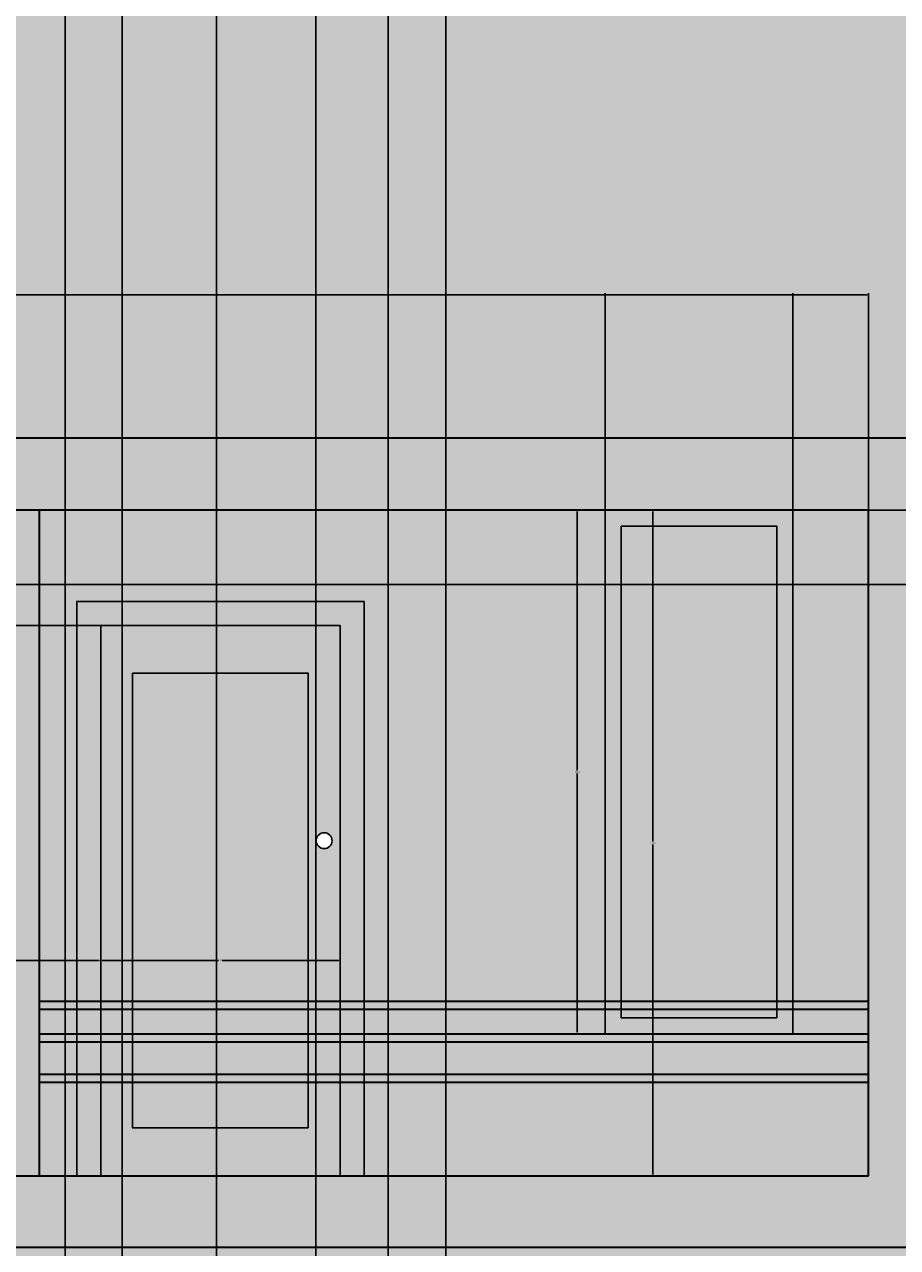
# Model space of a CAD drawing. Units: inches. Extents: x 73 to 607, y 92 to 651.
# Tile 15 of 18: x 337 to 446, y 311 to 465. Entities that reach past the tile are written whole.
import ezdxf

# ---------------------------------------------------------------- set-up
doc = ezdxf.new("R2010")
doc.units = ezdxf.units.IN
doc.header["$MEASUREMENT"] = 0
for name, color, linetype, lineweight in [('A-ANNO-DIMS', 2, 'Continuous', 18), ('A-DOOR', 3, 'Continuous', 25), ('A-ELEV', 7, 'Continuous', 35), ('A-ELEV-PATT-BKGD', 252, 'Continuous', 13), ('A-ELEV-PATT-FRAM', 38, 'Continuous', 13), ('A-ELEV-PATT-SHAD', 8, 'Continuous', 13), ('A-ELEV-PATT-WALL', 254, 'Continuous', 13), ('A-GLAZ', 4, 'Continuous', 25), ('A-GLAZ-PATT', 7, 'Continuous', 13)]:
    doc.layers.add(name, color=color, linetype=linetype, lineweight=lineweight)
doc.styles.get("Standard").update_dxf_attribs({"font": 'arial.ttf'})
doc.dimstyles.get("Standard").update_dxf_attribs({"dimtxt": 0.18, "dimasz": 0.18, "dimexe": 0.18, "dimexo": 0.0625, "dimgap": 0.09, "dimtad": 0, "dimtih": 1, "dimtoh": 1, "dimdec": 4, "dimzin": 0, "dimdsep": 46, "dimtxsty": 'Standard', "dimcen": 0.09, "dimadec": 0, "dimazin": 0, "dimtfac": 1, "dimtdec": 4, "dimtofl": 0, "dimtmove": 0, "dimatfit": 3, "dimfxl": 1, "dimtolj": 1, "dimtzin": 0, "dimarcsym": 0})

# ---------------------------------------------------------------- blocks, each defined once
blk = doc.blocks.new('*U3')
blk.add_lwpolyline([(3.12, 0.01), (0.12, 0.01), (0.12, 72.01), (36.12, 72.01), (36.12, 0.01), (33.12, 0.01)])
for points in [[(33.12, 68.99), (33.12, 0.01), (3.12, 0.01), (3.12, 68.99)], [(29.12, 6.01), (29.12, 62.99), (7.12, 62.99), (7.12, 6.01)]]:
    blk.add_lwpolyline(points, close=True)
blk.add_circle((31.12, 42.01), 1)
blk = doc.blocks.new('*D52')
at = {"layer": 'A-ANNO-DIMS', "color": 0, "lineweight": -2, "transparency": 16777216}
for p, q in [((206.13, 403.7), (206.13, 430.82)), ((442.52, 403.7), (442.52, 430.82)), ((206.31, 430.64), (323.93, 430.64)), ((442.34, 430.64), (324.72, 430.64))]:
    blk.add_line(p, q, dxfattribs=at)
at = {"layer": 'A-ANNO-DIMS', "color": 0, "transparency": 16777216}
for points in [[(206.31, 430.67), (206.31, 430.61), (206.13, 430.64)], [(442.34, 430.67), (442.34, 430.61), (442.52, 430.64)]]:
    blk.add_solid(points, dxfattribs=at)
at = {"layer": 'Defpoints', "color": 0, "transparency": 16777216}
for p in [(442.52, 430.64), (206.13, 403.64), (442.52, 403.64)]:
    blk.add_point(p, dxfattribs=at)
at = {"layer": 'A-ANNO-DIMS', "color": 0, "transparency": 16777216, "insert": (324.33, 430.64), "char_height": 0.18, "attachment_point": 5}
blk.add_mtext('\\A1;236.4', dxfattribs=at)
blk = doc.blocks.new('*D53')
at = {"layer": 'A-ANNO-DIMS', "color": 0, "lineweight": -2, "transparency": 16777216}
for p, q in [((442.46, 403.64), (415.34, 403.64)), ((415.52, 403.46), (415.52, 362.1)), ((415.52, 320.38), (415.52, 361.74)), ((442.46, 320.2), (415.34, 320.2))]:
    blk.add_line(p, q, dxfattribs=at)
at = {"layer": 'A-ANNO-DIMS', "color": 0, "transparency": 16777216}
for points in [[(415.49, 403.46), (415.55, 403.46), (415.52, 403.64)], [(415.49, 320.38), (415.55, 320.38), (415.52, 320.2)]]:
    blk.add_solid(points, dxfattribs=at)
at = {"layer": 'Defpoints', "color": 0, "transparency": 16777216}
for p in [(415.52, 403.64), (442.52, 403.64), (442.52, 320.2)]:
    blk.add_point(p, dxfattribs=at)
at = {"layer": 'A-ANNO-DIMS', "color": 0, "transparency": 16777216, "insert": (415.52, 361.92), "char_height": 0.18, "attachment_point": 5}
blk.add_mtext('\\A1;83.43', dxfattribs=at)
blk = doc.blocks.new('*D54')
at = {"layer": 'A-ANNO-DIMS', "color": 0, "lineweight": -2, "transparency": 16777216}
for p, q in [((206.13, 320.27), (206.13, 347.38)), ((206.31, 347.2), (275.84, 347.2)), ((346.14, 347.2), (276.61, 347.2)), ((346.32, 320.27), (346.32, 347.38))]:
    blk.add_line(p, q, dxfattribs=at)
at = {"layer": 'A-ANNO-DIMS', "color": 0, "transparency": 16777216}
for points in [[(206.31, 347.23), (206.31, 347.17), (206.13, 347.2)], [(346.14, 347.23), (346.14, 347.17), (346.32, 347.2)]]:
    blk.add_solid(points, dxfattribs=at)
at = {"layer": 'Defpoints', "color": 0, "transparency": 16777216}
for p in [(346.32, 347.2), (206.13, 320.2), (346.32, 320.2)]:
    blk.add_point(p, dxfattribs=at)
at = {"layer": 'A-ANNO-DIMS', "color": 0, "transparency": 16777216, "insert": (276.23, 347.2), "char_height": 0.18, "attachment_point": 5}
blk.add_mtext('\\A1;140.2', dxfattribs=at)
blk = doc.blocks.new('*D55')
at = {"layer": 'A-ANNO-DIMS', "color": 0, "lineweight": -2, "transparency": 16777216}
for p, q in [((346.32, 320.27), (346.32, 347.38)), ((346.5, 347.2), (361.1, 347.2)), ((376.14, 347.2), (361.54, 347.2)), ((376.32, 320.27), (376.32, 347.38))]:
    blk.add_line(p, q, dxfattribs=at)
at = {"layer": 'A-ANNO-DIMS', "color": 0, "transparency": 16777216}
for points in [[(346.5, 347.23), (346.5, 347.17), (346.32, 347.2)], [(376.14, 347.23), (376.14, 347.17), (376.32, 347.2)]]:
    blk.add_solid(points, dxfattribs=at)
at = {"layer": 'Defpoints', "color": 0, "transparency": 16777216}
for p in [(376.32, 347.2), (346.32, 320.2), (376.32, 320.2)]:
    blk.add_point(p, dxfattribs=at)
at = {"layer": 'A-ANNO-DIMS', "color": 0, "transparency": 16777216, "insert": (361.32, 347.2), "char_height": 0.18, "attachment_point": 5}
blk.add_mtext('\\A1;30', dxfattribs=at)
blk = doc.blocks.new('*D56')
at = {"layer": 'A-ANNO-DIMS', "color": 0, "lineweight": -2, "transparency": 16777216}
for p, q in [((346.26, 389.18), (319.14, 389.18)), ((319.32, 389), (319.32, 354.87)), ((319.32, 320.38), (319.32, 354.51)), ((346.26, 320.2), (319.14, 320.2))]:
    blk.add_line(p, q, dxfattribs=at)
at = {"layer": 'A-ANNO-DIMS', "color": 0, "transparency": 16777216}
for points in [[(319.29, 389), (319.35, 389), (319.32, 389.18)], [(319.29, 320.38), (319.35, 320.38), (319.32, 320.2)]]:
    blk.add_solid(points, dxfattribs=at)
at = {"layer": 'Defpoints', "color": 0, "transparency": 16777216}
for p in [(319.32, 389.18), (346.32, 389.18), (346.32, 320.2)]:
    blk.add_point(p, dxfattribs=at)
at = {"layer": 'A-ANNO-DIMS', "color": 0, "transparency": 16777216, "insert": (319.32, 354.69), "char_height": 0.18, "attachment_point": 5}
blk.add_mtext('\\A1;68.98', dxfattribs=at)
blk = doc.blocks.new('*D57')
at = {"layer": 'A-ANNO-DIMS', "color": 0, "lineweight": -2, "transparency": 16777216}
for p, q in [((409.52, 403.7), (409.52, 430.82)), ((433.03, 403.7), (433.03, 430.82)), ((409.7, 430.64), (420.89, 430.64)), ((432.85, 430.64), (421.65, 430.64))]:
    blk.add_line(p, q, dxfattribs=at)
at = {"layer": 'A-ANNO-DIMS', "color": 0, "transparency": 16777216}
for points in [[(409.7, 430.67), (409.7, 430.61), (409.52, 430.64)], [(432.85, 430.67), (432.85, 430.61), (433.03, 430.64)]]:
    blk.add_solid(points, dxfattribs=at)
at = {"layer": 'Defpoints', "color": 0, "transparency": 16777216}
for p in [(433.03, 430.64), (409.52, 403.64), (433.03, 403.64)]:
    blk.add_point(p, dxfattribs=at)
at = {"layer": 'A-ANNO-DIMS', "color": 0, "transparency": 16777216, "insert": (421.27, 430.64), "char_height": 0.18, "attachment_point": 5}
blk.add_mtext('\\A1;23.51', dxfattribs=at)
blk = doc.blocks.new('*D58')
at = {"layer": 'A-ANNO-DIMS', "color": 0, "lineweight": -2, "transparency": 16777216}
for p, q in [((432.96, 403.64), (405.85, 403.64)), ((406.03, 403.46), (406.03, 371)), ((406.03, 338.18), (406.03, 370.64)), ((432.96, 338), (405.85, 338))]:
    blk.add_line(p, q, dxfattribs=at)
at = {"layer": 'A-ANNO-DIMS', "color": 0, "transparency": 16777216}
for points in [[(406, 403.46), (406.06, 403.46), (406.03, 403.64)], [(406, 338.18), (406.06, 338.18), (406.03, 338)]]:
    blk.add_solid(points, dxfattribs=at)
at = {"layer": 'Defpoints', "color": 0, "transparency": 16777216}
for p in [(406.03, 403.64), (433.03, 403.64), (433.03, 338)]:
    blk.add_point(p, dxfattribs=at)
at = {"layer": 'A-ANNO-DIMS', "color": 0, "transparency": 16777216, "insert": (406.03, 370.82), "char_height": 0.18, "attachment_point": 5}
blk.add_mtext('\\A1;65.63', dxfattribs=at)
blk = doc.blocks.new('*D79')
at = {"layer": 'A-ANNO-DIMS', "color": 0, "lineweight": -2, "transparency": 16777216}
for p, q in [((334.73, 403.64), (607.28, 403.64)), ((607.1, 403.46), (607.1, 399.16)), ((607.1, 394.49), (607.1, 398.79)), ((316.35, 394.31), (607.28, 394.31))]:
    blk.add_line(p, q, dxfattribs=at)
at = {"layer": 'A-ANNO-DIMS', "color": 0, "transparency": 16777216}
for points in [[(607.07, 403.46), (607.13, 403.46), (607.1, 403.64)], [(607.07, 394.49), (607.13, 394.49), (607.1, 394.31)]]:
    blk.add_solid(points, dxfattribs=at)
at = {"layer": 'Defpoints', "color": 0, "transparency": 16777216}
for p in [(334.67, 403.64), (316.28, 394.31), (607.1, 394.31)]:
    blk.add_point(p, dxfattribs=at)
at = {"layer": 'A-ANNO-DIMS', "color": 0, "transparency": 16777216, "insert": (607.1, 398.98), "char_height": 0.18, "attachment_point": 5}
blk.add_mtext('\\A1;9.322', dxfattribs=at)
blk = doc.blocks.new('*D81')
at = {"layer": 'A-ANNO-DIMS', "color": 0, "lineweight": -2, "transparency": 16777216}
for p, q in [((341.87, 247.47), (341.87, 650.98)), ((342.05, 650.8), (345.04, 650.8)), ((348.82, 650.8), (345.83, 650.8)), ((349, 237.52), (349, 650.98))]:
    blk.add_line(p, q, dxfattribs=at)
at = {"layer": 'A-ANNO-DIMS', "color": 0, "transparency": 16777216}
for points in [[(342.05, 650.83), (342.05, 650.77), (341.87, 650.8)], [(348.82, 650.83), (348.82, 650.77), (349, 650.8)]]:
    blk.add_solid(points, dxfattribs=at)
at = {"layer": 'Defpoints', "color": 0, "transparency": 16777216}
for p in [(349, 650.8), (341.87, 247.41), (349, 237.45)]:
    blk.add_point(p, dxfattribs=at)
at = {"layer": 'A-ANNO-DIMS', "color": 0, "transparency": 16777216, "insert": (345.43, 650.8), "char_height": 0.18, "attachment_point": 5}
blk.add_mtext('\\A1;7.128', dxfattribs=at)
blk = doc.blocks.new('*D82')
at = {"layer": 'A-ANNO-DIMS', "color": 0, "lineweight": -2, "transparency": 16777216}
for p, q in [((349, 237.52), (349, 650.98)), ((349.18, 650.8), (354.47, 650.8)), ((360.67, 650.8), (355.38, 650.8)), ((360.85, 239), (360.85, 650.98))]:
    blk.add_line(p, q, dxfattribs=at)
at = {"layer": 'A-ANNO-DIMS', "color": 0, "transparency": 16777216}
for points in [[(349.18, 650.83), (349.18, 650.77), (349, 650.8)], [(360.67, 650.83), (360.67, 650.77), (360.85, 650.8)]]:
    blk.add_solid(points, dxfattribs=at)
at = {"layer": 'Defpoints', "color": 0, "transparency": 16777216}
for p in [(360.85, 650.8), (360.85, 238.93), (349, 237.45)]:
    blk.add_point(p, dxfattribs=at)
at = {"layer": 'A-ANNO-DIMS', "color": 0, "transparency": 16777216, "insert": (354.92, 650.8), "char_height": 0.18, "attachment_point": 5}
blk.add_mtext('\\A1;11.852', dxfattribs=at)
blk = doc.blocks.new('*D83')
at = {"layer": 'A-ANNO-DIMS', "color": 0, "lineweight": -2, "transparency": 16777216}
for p, q in [((360.85, 239), (360.85, 650.98)), ((361.03, 650.8), (366.6, 650.8)), ((373.08, 650.8), (367.51, 650.8)), ((373.26, 231.41), (373.26, 650.98))]:
    blk.add_line(p, q, dxfattribs=at)
at = {"layer": 'A-ANNO-DIMS', "color": 0, "transparency": 16777216}
for points in [[(361.03, 650.83), (361.03, 650.77), (360.85, 650.8)], [(373.08, 650.83), (373.08, 650.77), (373.26, 650.8)]]:
    blk.add_solid(points, dxfattribs=at)
at = {"layer": 'Defpoints', "color": 0, "transparency": 16777216}
for p in [(373.26, 650.8), (360.85, 238.93), (373.26, 231.35)]:
    blk.add_point(p, dxfattribs=at)
at = {"layer": 'A-ANNO-DIMS', "color": 0, "transparency": 16777216, "insert": (367.05, 650.8), "char_height": 0.18, "attachment_point": 5}
blk.add_mtext('\\A1;12.408', dxfattribs=at)
blk = doc.blocks.new('*D84')
at = {"layer": 'A-ANNO-DIMS', "color": 0, "lineweight": -2, "transparency": 16777216}
for p, q in [((373.26, 231.41), (373.26, 650.98)), ((373.44, 650.8), (377.4, 650.8)), ((382.15, 650.8), (378.19, 650.8)), ((382.33, 241.03), (382.33, 650.98))]:
    blk.add_line(p, q, dxfattribs=at)
at = {"layer": 'A-ANNO-DIMS', "color": 0, "transparency": 16777216}
for points in [[(373.44, 650.83), (373.44, 650.77), (373.26, 650.8)], [(382.15, 650.83), (382.15, 650.77), (382.33, 650.8)]]:
    blk.add_solid(points, dxfattribs=at)
at = {"layer": 'Defpoints', "color": 0, "transparency": 16777216}
for p in [(382.33, 650.8), (382.33, 240.97), (373.26, 231.35)]:
    blk.add_point(p, dxfattribs=at)
at = {"layer": 'A-ANNO-DIMS', "color": 0, "transparency": 16777216, "insert": (377.79, 650.8), "char_height": 0.18, "attachment_point": 5}
blk.add_mtext('\\A1;9.074', dxfattribs=at)
blk = doc.blocks.new('*D85')
at = {"layer": 'A-ANNO-DIMS', "color": 0, "lineweight": -2, "transparency": 16777216}
for p, q in [((382.33, 241.03), (382.33, 650.98)), ((382.51, 650.8), (385.55, 650.8)), ((389.37, 650.8), (386.33, 650.8)), ((389.55, 232.52), (389.55, 650.98))]:
    blk.add_line(p, q, dxfattribs=at)
at = {"layer": 'A-ANNO-DIMS', "color": 0, "transparency": 16777216}
for points in [[(382.51, 650.83), (382.51, 650.77), (382.33, 650.8)], [(389.37, 650.83), (389.37, 650.77), (389.55, 650.8)]]:
    blk.add_solid(points, dxfattribs=at)
at = {"layer": 'Defpoints', "color": 0, "transparency": 16777216}
for p in [(389.55, 650.8), (382.33, 240.97), (389.55, 232.46)]:
    blk.add_point(p, dxfattribs=at)
at = {"layer": 'A-ANNO-DIMS', "color": 0, "transparency": 16777216, "insert": (385.94, 650.8), "char_height": 0.18, "attachment_point": 5}
blk.add_mtext('\\A1;7.222', dxfattribs=at)

msp = doc.modelspace()

# ---------------------------------------------------------------- hatches: boundary and pattern name
at = {"layer": 'A-ELEV-PATT-BKGD'}
h = msp.add_hatch(color=256, dxfattribs=at)
h.dxf.hatch_style = 1
h.paths.add_polyline_path([(321.3008, 479.2042), (312.3008, 479.2042), (312.3008, 478.7576), (312.3008, 412.636), (321.3008, 412.636)])
h.paths.add_polyline_path([(312.3008, 504.7576), (256.4726, 504.7576), (256.4726, 503.4576), (312.3008, 503.4576)], flags=17)
h.paths.add_polyline_path([(321.3008, 543.1576), (321.3008, 552.1576), (320.3257, 552.1576), (312.3008, 552.1576), (256.4726, 552.1576), (256.4726, 543.1576), (312.3008, 543.1576), (312.3008, 479.2042), (321.3008, 479.2042)])
h.paths.add_polyline_path([(451.5214, 412.636), (256.4726, 412.636), (256.4726, 403.636), (442.5214, 403.636), (442.5214, 320.2042), (206.1343, 320.2042), (206.1343, 320.9135), (206.1343, 403.636), (256.4726, 403.636), (256.4726, 412.636), (201.6343, 412.636), (201.6343, 320.9135), (201.6343, 320.2042), (201.6343, 311.2042), (256.4726, 311.2042), (451.5214, 311.2042)])
h.paths.add_polyline_path([(431.07, 258.6914), (369.5339, 258.6914), (369.5339, 247.4054), (396.692, 247.4054), (425.07, 247.4054), (425.07, 194.7312), (396.692, 194.6197), (396.692, 194.5366), (369.5339, 194.5366), (369.5339, 185.6619), (431.07, 185.6619)])
h.paths.add_polyline_path([(580.0983, 262.3024), (451.5214, 262.3024), (451.5214, 143.2042), (580.0983, 143.2042)])
h.paths.add_polyline_path([(454.7049, 174.802), (454.7049, 256.6321), (577.9249, 256.6321), (577.9249, 174.802)], flags=16)
h.paths.add_polyline_path([(465.9716, 191.1416, -1), (473.7874, 191.1416, -1)], flags=0)
h.paths.add_polyline_path([(490.5373, 181.6586, -1), (494.9999, 181.6586, -1)], flags=0)
h.paths.add_polyline_path([(476.2996, 209.8287, -1), (500.5844, 209.8287, -1)], flags=0)
h.paths.add_polyline_path([(505.3326, 194.7675, -1), (512.5843, 194.7675, -1)], flags=0)
h.paths.add_polyline_path([(520.9613, 186.679, -1), (526.544, 186.679, -1)], flags=0)
h.paths.add_polyline_path([(466.8103, 225.7267, -1), (470.1573, 225.7267, -1)], flags=0)
h.paths.add_polyline_path([(527.1059, 203.6926, -1), (536.0311, 203.6926, -1)], flags=0)
h.paths.add_polyline_path([(504.775, 232.6995, -1), (513.7002, 232.6995, -1)], flags=0)
h.paths.add_polyline_path([(546.9241, 183.611, -1), (554.7336, 183.611, -1)], flags=0)
h.paths.add_polyline_path([(459.5544, 243.856, -1), (466.8061, 243.856, -1)], flags=0)
h.paths.add_polyline_path([(476.3045, 246.924, -1), (488.5767, 246.924, -1)], flags=0)
h.paths.add_polyline_path([(529.9044, 226.8424, -1), (556.68, 226.8424, -1)], flags=0)
h.paths.add_polyline_path([(554.1814, 203.9716, -1), (561.4331, 203.9716, -1)], flags=0)
h.paths.add_polyline_path([(567.8561, 193.3729, -1), (570.6475, 193.3729, -1)], flags=0)
h.paths.add_polyline_path([(522.3584, 250.271, -1), (525.7053, 250.271, -1)], flags=0)
h.paths.add_polyline_path([(561.9965, 245.2506, -1), (567.5748, 245.2506, -1)], flags=0)
h.paths.add_polyline_path([(347.8686, 194.5366), (341.8686, 194.5366), (341.8686, 194.5452), (314.0144, 194.5452), (314.0144, 188.5452), (347.8686, 188.5452)])
h.paths.add_polyline_path([(347.8686, 253.4054), (314.0144, 253.4054), (314.0144, 247.4054), (341.8686, 247.4054), (347.8686, 247.4054)])
h.paths.add_polyline_path([(304.3559, 253.4054), (298.3559, 253.4054), (298.3559, 188.5452), (304.3559, 188.5452)])
h.paths.add_polyline_path([(450.6603, 552.1576), (369.9727, 552.1576), (369.9727, 479.2042), (374.4727, 479.2042), (374.4727, 547.6576), (446.1603, 547.6576), (446.1603, 479.2042), (450.6603, 479.2042)])
h.paths.add_polyline_path([(374.4727, 479.2042), (369.9727, 479.2042), (369.9727, 465.0632), (374.4727, 465.0632)])
h.paths.add_polyline_path([(450.6603, 479.2042), (446.1603, 479.2042), (446.1603, 465.0632), (450.6603, 465.0632)])
h.paths.add_polyline_path([(256.4726, 281.6039), (109.0983, 281.6039), (100.0983, 281.6039), (100.0983, 167.2042), (100.0983, 143.2042), (109.0983, 143.2042), (109.0983, 167.2042), (109.0983, 272.6039), (256.4726, 272.6039)])
at = {"layer": 'A-ELEV-PATT-FRAM'}
h = msp.add_hatch(color=256, dxfattribs=at)
h.dxf.hatch_style = 1
h.paths.add_polyline_path([(433.025, 403.636), (409.515, 403.636), (409.515, 342.1009), (411.515, 342.1009), (411.515, 401.636), (431.025, 401.636), (431.025, 342.1009), (433.025, 342.1009)])
h.paths.add_polyline_path([(433.025, 341.1009), (431.025, 341.1009), (431.025, 340.0025), (411.515, 340.0025), (411.515, 341.1009), (409.515, 341.1009), (409.515, 338.0025), (433.025, 338.0025)])
h.paths.add_polyline_path([(425.07, 247.4054), (396.692, 247.4054), (396.692, 194.6197), (425.07, 194.7312)])
h.paths.add_polyline_path([(423.07, 245.4054), (423.07, 196.7234), (398.8836, 196.6284), (398.692, 245.4054)], flags=16)
h.paths.add_polyline_path([(341.8686, 247.4054), (314.0144, 247.4054), (314.0144, 245.4054), (339.8686, 245.4054), (339.8686, 196.5452), (314.0144, 196.5452), (314.0144, 194.5452), (341.8686, 194.5452)])
h.paths.add_polyline_path([(372.3213, 383.1812), (350.3213, 383.1812), (350.3213, 342.1009), (372.3213, 342.1009)], flags=16)
h.paths.add_polyline_path([(376.3213, 389.1812), (346.3213, 389.1812), (346.3213, 342.1009), (350.3213, 342.1009), (350.3213, 383.1812), (372.3213, 383.1812), (372.3213, 342.1009), (376.3213, 342.1009)], flags=17)
h.paths.add_polyline_path([(375.3213, 362.2042, -1), (373.3213, 362.2042, -1)], flags=16)
h.paths.add_polyline_path([(379.3213, 392.2042), (343.3213, 392.2042), (343.3213, 342.1009), (346.3213, 342.1009), (346.3213, 389.1812), (376.3213, 389.1812), (376.3213, 342.1009), (379.3213, 342.1009)])
h.paths.add_polyline_path([(350.3213, 341.1009), (346.3213, 341.1009), (346.3213, 338.0025), (350.3213, 338.0025)])
h.paths.add_polyline_path([(346.3213, 341.1009), (343.3213, 341.1009), (343.3213, 338.0025), (346.3213, 338.0025)])
h.paths.add_polyline_path([(346.3213, 337.0025), (343.3213, 337.0025), (343.3213, 332.9397), (346.3213, 332.9397)])
h.paths.add_polyline_path([(350.3213, 337.0025), (346.3213, 337.0025), (346.3213, 332.9397), (350.3213, 332.9397)])
h.paths.add_polyline_path([(350.3213, 331.9397), (346.3213, 331.9397), (346.3213, 320.2042), (376.3213, 320.2042), (376.3213, 331.9397), (372.3213, 331.9397), (372.3213, 326.2042), (350.3213, 326.2042)])
h.paths.add_polyline_path([(372.3213, 337.0025), (350.3213, 337.0025), (350.3213, 332.9397), (372.3213, 332.9397)])
h.paths.add_polyline_path([(372.3213, 341.1009), (350.3213, 341.1009), (350.3213, 338.0025), (372.3213, 338.0025)])
h.paths.add_polyline_path([(376.3213, 341.1009), (372.3213, 341.1009), (372.3213, 338.0025), (376.3213, 338.0025)])
h.paths.add_polyline_path([(376.3213, 337.0025), (372.3213, 337.0025), (372.3213, 332.9397), (376.3213, 332.9397)])
h.paths.add_polyline_path([(379.3213, 341.1009), (376.3213, 341.1009), (376.3213, 338.0025), (379.3213, 338.0025)])
h.paths.add_polyline_path([(379.3213, 337.0025), (376.3213, 337.0025), (376.3213, 332.9397), (379.3213, 332.9397)])
h.paths.add_polyline_path([(379.3213, 331.9397), (376.3213, 331.9397), (376.3213, 320.2042), (379.3213, 320.2042)])
h.paths.add_polyline_path([(372.3213, 331.9397), (350.3213, 331.9397), (350.3213, 326.2042), (372.3213, 326.2042)], flags=17)
h.paths.add_polyline_path([(346.3213, 331.9397), (343.3213, 331.9397), (343.3213, 320.2042), (346.3213, 320.2042)])
at = {"layer": 'A-ELEV-PATT-SHAD'}
h = msp.add_hatch(color=256, dxfattribs=at)
h.dxf.hatch_style = 1
h.paths.add_polyline_path([(451.5214, 412.636), (256.4726, 412.636), (256.4726, 403.636), (442.5214, 403.636), (442.5214, 320.2042), (206.1343, 320.2042), (206.1343, 320.9135), (206.1343, 403.636), (256.4726, 403.636), (256.4726, 412.636), (201.6343, 412.636), (201.6343, 320.9135), (201.6343, 320.2042), (201.6343, 311.2042), (256.4726, 311.2042), (451.5214, 311.2042)])
h.paths.add_polyline_path([(580.0983, 262.3024), (451.5214, 262.3024), (451.5214, 143.2042), (580.0983, 143.2042)])
h.paths.add_polyline_path([(454.7049, 174.802), (454.7049, 256.6321), (577.9249, 256.6321), (577.9249, 174.802)], flags=16)
h.paths.add_polyline_path([(465.9716, 191.1416, -1), (473.7874, 191.1416, -1)], flags=0)
h.paths.add_polyline_path([(490.5373, 181.6586, -1), (494.9999, 181.6586, -1)], flags=0)
h.paths.add_polyline_path([(476.2996, 209.8287, -1), (500.5844, 209.8287, -1)], flags=0)
h.paths.add_polyline_path([(505.3326, 194.7675, -1), (512.5843, 194.7675, -1)], flags=0)
h.paths.add_polyline_path([(520.9613, 186.679, -1), (526.544, 186.679, -1)], flags=0)
h.paths.add_polyline_path([(466.8103, 225.7267, -1), (470.1573, 225.7267, -1)], flags=0)
h.paths.add_polyline_path([(527.1059, 203.6926, -1), (536.0311, 203.6926, -1)], flags=0)
h.paths.add_polyline_path([(459.5544, 243.856, -1), (466.8061, 243.856, -1)], flags=0)
h.paths.add_polyline_path([(504.775, 232.6995, -1), (513.7002, 232.6995, -1)], flags=0)
h.paths.add_polyline_path([(476.3045, 246.924, -1), (488.5767, 246.924, -1)], flags=0)
h.paths.add_polyline_path([(546.9241, 183.611, -1), (554.7336, 183.611, -1)], flags=0)
h.paths.add_polyline_path([(529.9044, 226.8424, -1), (556.68, 226.8424, -1)], flags=0)
h.paths.add_polyline_path([(554.1814, 203.9716, -1), (561.4331, 203.9716, -1)], flags=0)
h.paths.add_polyline_path([(522.3584, 250.271, -1), (525.7053, 250.271, -1)], flags=0)
h.paths.add_polyline_path([(567.8561, 193.3729, -1), (570.6475, 193.3729, -1)], flags=0)
h.paths.add_polyline_path([(561.9965, 245.2506, -1), (567.5748, 245.2506, -1)], flags=0)
h.paths.add_polyline_path([(431.07, 258.6914), (369.5339, 258.6914), (369.5339, 247.4054), (396.692, 247.4054), (425.07, 247.4054), (425.07, 194.7312), (396.692, 194.6197), (396.692, 194.5366), (369.5339, 194.5366), (369.5339, 185.6619), (431.07, 185.6619)])
h.paths.add_polyline_path([(347.8686, 253.4054), (314.0144, 253.4054), (314.0144, 247.4054), (341.8686, 247.4054), (347.8686, 247.4054)])
h.paths.add_polyline_path([(304.3559, 253.4054), (298.3559, 253.4054), (298.3559, 188.5452), (304.3559, 188.5452)])
h.paths.add_polyline_path([(347.8686, 194.5366), (341.8686, 194.5366), (341.8686, 194.5452), (314.0144, 194.5452), (314.0144, 188.5452), (347.8686, 188.5452)])
h = msp.add_hatch(color=256, dxfattribs=at)
h.dxf.hatch_style = 1
h.paths.add_polyline_path([(338.6695, 403.636), (334.6695, 403.636), (334.6695, 320.2042), (338.6695, 320.2042)])
at = {"layer": 'A-ELEV-PATT-WALL'}
h = msp.add_hatch(color=256, dxfattribs=at)
h.dxf.hatch_style = 1
h.paths.add_polyline_path([(509.9692, 483.857), (450.6603, 483.857), (450.6603, 465.0632), (446.1603, 465.0632), (446.1603, 484.2142), (374.4727, 484.2142), (374.4727, 465.0632), (369.9727, 465.0632), (369.9727, 484.2142), (321.3008, 484.2142), (321.3008, 412.636), (451.5214, 412.636), (451.5214, 311.2042), (314.0144, 311.2042), (314.0144, 253.4054), (347.8686, 253.4054), (347.8686, 247.4054), (369.5339, 247.4054), (369.5339, 258.6914), (431.07, 258.6914), (431.07, 185.6619), (369.5339, 185.6619), (369.5339, 194.5366), (347.8686, 194.5366), (347.8686, 188.5452), (314.0144, 188.5452), (314.0144, 143.2042), (451.5214, 143.2042), (451.5214, 262.3024), (580.0983, 262.3024), (580.0983, 311.2042), (509.9692, 311.2042)])
h.paths.add_polyline_path([(304.3559, 311.2042), (256.4726, 311.2042), (256.4726, 167.2042), (256.4726, 143.2042), (304.3559, 143.2042), (304.3559, 188.5452), (298.3559, 188.5452), (298.3559, 253.4054), (304.3559, 253.4054)])
h = msp.add_hatch(color=256, dxfattribs=at)
h.dxf.hatch_style = 1
h.paths.add_polyline_path([(409.515, 403.636), (338.6695, 403.636), (338.6695, 342.1009), (343.3213, 342.1009), (343.3213, 392.2042), (379.3213, 392.2042), (379.3213, 342.1009), (409.515, 342.1009)])
h.paths.add_polyline_path([(442.5214, 331.9397), (379.3213, 331.9397), (379.3213, 320.2042), (442.5214, 320.2042)])
h.paths.add_polyline_path([(442.5214, 337.0025), (379.3213, 337.0025), (379.3213, 332.9397), (442.5214, 332.9397)])
h.paths.add_polyline_path([(409.515, 341.1009), (379.3213, 341.1009), (379.3213, 338.0025), (409.515, 338.0025)])
h.paths.add_polyline_path([(442.5214, 403.636), (433.025, 403.636), (433.025, 342.1009), (442.5214, 342.1009)])
h.paths.add_polyline_path([(442.5214, 341.1009), (433.025, 341.1009), (433.025, 338.0025), (442.5214, 338.0025)])
h.paths.add_polyline_path([(343.3213, 341.1009), (338.6695, 341.1009), (338.6695, 338.0025), (343.3213, 338.0025)])
h.paths.add_polyline_path([(343.3213, 337.0025), (338.6695, 337.0025), (338.6695, 332.9397), (343.3213, 332.9397)])
h.paths.add_polyline_path([(343.3213, 331.9397), (338.6695, 331.9397), (338.6695, 320.2042), (343.3213, 320.2042)])
at = {"layer": 'A-GLAZ-PATT'}
h = msp.add_hatch(color=256, dxfattribs=at)
h.dxf.hatch_style = 1
h.paths.add_polyline_path([(369.9727, 496.6899), (321.3008, 496.6899), (321.3008, 495.6899), (369.9727, 495.6899)])
h.paths.add_polyline_path([(394.7799, 496.6899), (374.4727, 496.6899), (374.4727, 495.6899), (394.7799, 495.6899)])
h.paths.add_polyline_path([(446.1603, 496.6899), (394.7799, 496.6899), (394.7799, 495.6899), (446.1603, 495.6899)])
h.paths.add_polyline_path([(446.1603, 504.2042), (394.7799, 504.2042), (394.7799, 503.2042), (446.1603, 503.2042)])
h.paths.add_polyline_path([(369.9727, 504.2042), (321.3008, 504.2042), (321.3008, 503.2042), (369.9727, 503.2042)])
h.paths.add_polyline_path([(394.7799, 504.2042), (374.4727, 504.2042), (374.4727, 503.2042), (394.7799, 503.2042)])
h.paths.add_polyline_path([(509.9692, 504.2042), (450.6603, 504.2042), (450.6603, 503.2042), (509.9692, 503.2042)])
h.paths.add_polyline_path([(509.9692, 496.6899), (450.6603, 496.6899), (450.6603, 495.6899), (509.9692, 495.6899)])
h.paths.add_polyline_path([(409.515, 342.1009), (338.6695, 342.1009), (338.6695, 341.1009), (409.515, 341.1009)])
h.paths.add_polyline_path([(442.5214, 338.0025), (338.6695, 338.0025), (338.6695, 337.0025), (442.5214, 337.0025)])
h.paths.add_polyline_path([(442.5214, 332.9397), (338.6695, 332.9397), (338.6695, 331.9397), (442.5214, 331.9397)])
h = msp.add_hatch(color=256, dxfattribs=at)
h.dxf.hatch_style = 1
h.set_gradient(color1=(0, 0, 255))
h.paths.add_polyline_path([(431.025, 401.636), (411.515, 401.636), (411.515, 342.1009), (431.025, 342.1009)])
h = msp.add_hatch(color=256, dxfattribs=at)
h.dxf.hatch_style = 1
h.paths.add_polyline_path([(411.515, 342.1009), (409.515, 342.1009), (409.515, 341.1009), (411.515, 341.1009)])
h.paths.add_polyline_path([(431.025, 342.1009), (411.515, 342.1009), (411.515, 341.1009), (431.025, 341.1009)])
h.paths.add_polyline_path([(433.025, 342.1009), (431.025, 342.1009), (431.025, 341.1009), (433.025, 341.1009)])
h.paths.add_polyline_path([(442.5214, 342.1009), (433.025, 342.1009), (433.025, 341.1009), (442.5214, 341.1009)])
h = msp.add_hatch(color=256, dxfattribs=at)
h.dxf.hatch_style = 1
h.set_gradient(color1=(0, 0, 255))
h.paths.add_polyline_path([(431.025, 341.1009), (411.515, 341.1009), (411.515, 340.0025), (431.025, 340.0025)])

# ---------------------------------------------------------------- linework, layer by layer
at = {"layer": 'A-ELEV'}
for p, q in [((451.5214, 412.636), (201.6343, 412.636)), ((442.5214, 403.636), (206.1343, 403.636)), ((338.6695, 320.2042), (338.6695, 403.636)), ((442.5214, 320.2042), (442.5214, 403.636)), ((338.6695, 342.1009), (442.5214, 342.1009)), ((338.6695, 341.1009), (442.5214, 341.1009)), ((338.6695, 338.0025), (442.5214, 338.0025)), ((338.6695, 337.0025), (442.5214, 337.0025)), ((338.6695, 332.9397), (442.5214, 332.9397)), ((338.6695, 331.9397), (442.5214, 331.9397)), ((206.1343, 320.2042), (442.5214, 320.2042)), ((451.5214, 311.2042), (256.4726, 311.2042))]:
    msp.add_line(p, q, dxfattribs=at)
at = {"layer": 'A-GLAZ'}
for points in [[(409.515, 403.636), (433.025, 403.636), (433.025, 338.0025), (409.515, 338.0025)], [(411.515, 401.636), (431.025, 401.636), (431.025, 340.0025), (411.515, 340.0025)]]:
    msp.add_lwpolyline(points, close=True, dxfattribs=at)

# ---------------------------------------------------------------- block references
at = {"layer": 'A-DOOR'}
msp.add_blockref('*U3', (343.1976, 320.1914), dxfattribs=at)

# ---------------------------------------------------------------- dimensions: what is measured, and where the dimension line sits
at = {"layer": 'A-ANNO-DIMS'}
for base, p1, p2, override, picture, middle in [((348.9968, 650.801), (341.8686, 247.4054), (348.9968, 237.4546), {"dimdec": 3, "dimlfac": 1, "dimrnd": 0, "dimzin": 0, "dimdsep": 46, "dimlunit": 2}, '*D81', (345.4327, 650.801)), ((360.8489, 650.801), (348.9968, 237.4546), (360.8489, 238.9349), {"dimdec": 3, "dimlfac": 1, "dimrnd": 0, "dimzin": 0, "dimdsep": 46, "dimlunit": 2}, '*D82', (354.9229, 650.801)), ((373.2566, 650.801), (360.8489, 238.9349), (373.2566, 231.3482), {"dimdec": 3, "dimlfac": 1, "dimrnd": 0, "dimzin": 0, "dimdsep": 46, "dimlunit": 2}, '*D83', (367.0527, 650.801)), ((382.3308, 650.801), (373.2566, 231.3482), (382.3308, 240.9703), {"dimdec": 3, "dimlfac": 1, "dimrnd": 0, "dimzin": 0, "dimdsep": 46, "dimlunit": 2}, '*D84', (377.7937, 650.801)), ((389.5532, 650.801), (382.3308, 240.9703), (389.5532, 232.4585), {"dimdec": 3, "dimlfac": 1, "dimrnd": 0, "dimzin": 0, "dimdsep": 46, "dimlunit": 2}, '*D85', (385.942, 650.801)), ((442.5214, 430.636), (206.1343, 403.636), (442.5214, 403.636), {"dimdec": 1, "dimlfac": 1, "dimrnd": 0, "dimzin": 0, "dimdsep": 46, "dimlunit": 2}, '*D52', (324.3278, 430.636)), ((433.025, 430.636), (409.515, 403.636), (433.025, 403.636), {"dimdec": 2, "dimlfac": 1, "dimrnd": 0, "dimzin": 0, "dimdsep": 46, "dimlunit": 2}, '*D57', (421.27, 430.636)), ((346.3213, 347.2042), (206.1343, 320.2042), (346.3213, 320.2042), {"dimdec": 1, "dimlfac": 1, "dimrnd": 0, "dimzin": 0, "dimdsep": 46, "dimlunit": 2}, '*D54', (276.2278, 347.2042)), ((376.3213, 347.2042), (346.3213, 320.2042), (376.3213, 320.2042), {"dimdec": 0, "dimlfac": 1, "dimrnd": 0, "dimzin": 0, "dimdsep": 46, "dimlunit": 2}, '*D55', (361.3213, 347.2042))]:
    dim = msp.add_linear_dim(base=base, p1=p1, p2=p2, dimstyle='Standard', override=override, dxfattribs=at)
    dim.commit()
    dim.dimension.update_dxf_attribs({"geometry": picture, "text_midpoint": middle})
for base, p1, p2, override, picture, middle in [((607.0983, 394.3141), (334.6695, 403.636), (316.2836, 394.3141), {"dimdec": 3, "dimlfac": 1, "dimrnd": 0, "dimzin": 0, "dimdsep": 46, "dimlunit": 2}, '*D79', (607.0983, 398.9751)), ((406.025, 403.636), (433.025, 338.0025), (433.025, 403.636), {"dimdec": 2, "dimlfac": 1, "dimrnd": 0, "dimzin": 0, "dimdsep": 46, "dimlunit": 2}, '*D58', (406.025, 370.8192)), ((415.5214, 403.636), (442.5214, 320.2042), (442.5214, 403.636), {"dimdec": 2, "dimlfac": 1, "dimrnd": 0, "dimzin": 0, "dimdsep": 46, "dimlunit": 2}, '*D53', (415.5214, 361.9201)), ((319.3213, 389.1812), (346.3213, 320.2042), (346.3213, 389.1812), {"dimdec": 2, "dimlfac": 1, "dimrnd": 0, "dimzin": 0, "dimdsep": 46, "dimlunit": 2}, '*D56', (319.3213, 354.6927))]:
    dim = msp.add_linear_dim(base=base, p1=p1, p2=p2, angle=90, dimstyle='Standard', override=override, dxfattribs=at)
    dim.commit()
    dim.dimension.update_dxf_attribs({"geometry": picture, "text_midpoint": middle})

doc.saveas('drawing.dxf')
